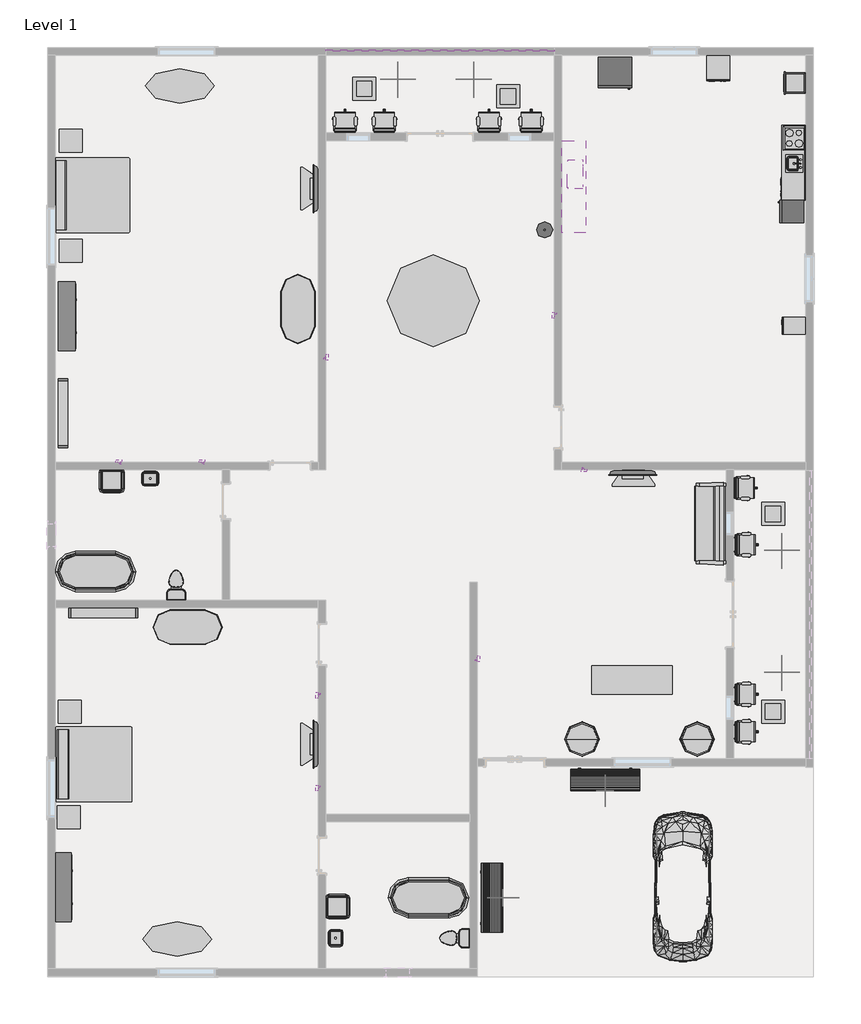
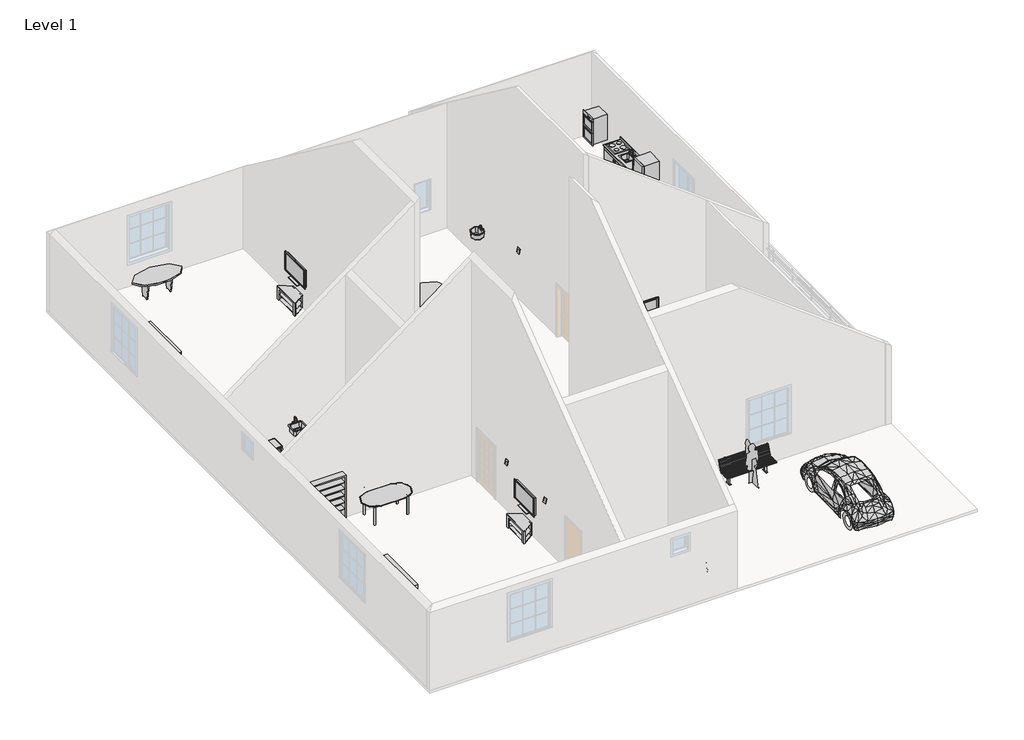
# One storey, part 2 of 2: 39 furniture elements, 20 proxies, 8 flow terminals, 8 geographic elements, 1 railing.
"""IFC4 building model written with IfcOpenShell, lengths in millimetres."""

from ifc_helpers import new_model, si_unit, point, frame, frame_2d, origin, place, context, project, spatial, circle_curve, trimmed, segment, composite_curve, outline, extrude, transform, mapped, element, save
from components import proxy_7e1014cc, proxy_a6faaae8, proxy_45b28599, proxy_19aded4c, kitchenette_medium_kitchenette_medium_844211aa, proxy_8a8d5ab2, proxy_8b8c2dc4, rpc_beetle_rpc_beetle_3ce7ba48, rpc_female_69e001fa, rpc_picture_frame_rpc_picture_frame_c25e3fe9, proxy_c523a7b7, proxy_9109806d, flow_terminal_871c2e40, flow_terminal_d49f872f, flow_terminal_62a433f7, toilet_domestic_3d_toilet_domestic_3d_f7549cf7, toilet_domestic_3d_toilet_domestic_3d_183bbd19, flow_terminal_b46ab875, furniture_1fc5af50, chair_task_arms_chair_task_arms_fa5a08ef, furniture_c6510c7c, counter_top_w_sink_hole_counter_top_w_sink_hole_22cae41e, furniture_7c473f12, furniture_c6fa4874, furniture_aff9b2fb, furniture_fdf74506, tv_stand_tv_stand_6ce107e5, furniture_b5c51a22, furniture_92191dda, furniture_2c34a4f9, furniture_5d3b8c6f, furniture_027a2ad9, furniture_5bc9ed15, furniture_c80d6d9c, geographic_element_235d1464, rpc_tree_conifer_chinese_juniper_7_1b9786cd, trash_can_trash_can_952d1acd

model = new_model("IFC4")

# Units and contexts
model_context = context("Model", 3, world=origin())
ifc_project = project(units=[si_unit("LENGTHUNIT", "METRE", prefix="MILLI")], contexts=[model_context])

# Site, building, storey
site = spatial("IfcSite", under=ifc_project)
building = spatial("IfcBuilding", under=site)
storey = spatial("IfcBuildingStorey", under=building, Name="Level 1", Elevation=0.0)

# Proxies
placement = place(None, origin())
proxy_shape = proxy_7e1014cc(model_context)
element("IfcBuildingElementProxy", 1, Name="18\" x 24\" x 34 1/2\"", ObjectType="18\" x 24\" x 34 1/2\"", at=placement, inside=storey, context=model_context, shape_type="MappedRepresentation", body=[
    mapped(proxy_shape, transform((4829.120864, 3840.6220575, 0.0), x_axis=(0.0, -1.0000000000000004, 0.0), y_axis=(1.0000000000000004, 0.0, 0.0), z_axis=(0.0, 0.0, 1.0))),
])
proxy_2_shape = proxy_a6faaae8(model_context)
element("IfcBuildingElementProxy", 2, Name="Cook Top-4 Unit2 : 22\" x 20\"", ObjectType="Cook Top-4 Unit2 : 22\" x 20\"", at=placement, inside=storey, context=model_context, shape_type="MappedRepresentation", body=[
    mapped(proxy_2_shape, transform((5095.5704288, 8500.2045891, 0.0), x_axis=(0.0, -1.0000000000000002, 0.0), y_axis=(1.0000000000000002, 0.0, 0.0), z_axis=(0.0, 0.0, 1.0))),
])
proxy_3_shape = proxy_45b28599(model_context)
element("IfcBuildingElementProxy", 3, Name="Dishwasher : 24\" x 24\" x 34\"", ObjectType="Dishwasher : 24\" x 24\" x 34\"", at=placement, inside=storey, context=model_context, shape_type="MappedRepresentation", body=[
    mapped(proxy_3_shape, transform((4803.720864, 7549.0220575, 0.0), x_axis=(0.0, -1.0000000000000002, 0.0), y_axis=(1.0000000000000002, 0.0, 0.0), z_axis=(0.0, 0.0, 1.0))),
])
proxy_4_shape = proxy_19aded4c(model_context)
element("IfcBuildingElementProxy", 4, Name="Dishwasher : 24\" x 26 1/4\" x 34 1/2\"", ObjectType="Dishwasher : 24\" x 26 1/4\" x 34 1/2\"", at=placement, inside=storey, context=model_context, shape_type="MappedRepresentation", body=[
    mapped(proxy_4_shape, transform((2706.6529603, 10068.9050243, 0.0), x_axis=(1.0, 0.0, 0.0), y_axis=(0.0, 1.0, 0.0), z_axis=(0.0, 0.0, 1.0))),
])
kitchenette_medium_kitchenette_medium_shape = kitchenette_medium_kitchenette_medium_844211aa(model_context)
element("IfcBuildingElementProxy", 5, Name="Kitchenette - Medium : Kitchenette - Medium", ObjectType="Kitchenette - Medium : Kitchenette - Medium", at=placement, inside=storey, context=model_context, shape_type="MappedRepresentation", body=[
    mapped(kitchenette_medium_kitchenette_medium_shape, transform((5400.3704288, 8176.042294, 0.0), x_axis=(0.0, -1.0000000000000002, 0.0), y_axis=(1.0000000000000002, 0.0, 0.0), z_axis=(0.0, 0.0, 1.0))),
])
proxy_5_shape = proxy_8a8d5ab2(model_context)
element("IfcBuildingElementProxy", 6, Name="Microwave : 30\" x 16\" x 18\"", ObjectType="Microwave : 30\" x 16\" x 18\"", at=placement, inside=storey, context=model_context, shape_type="MappedRepresentation", body=[
    mapped(proxy_5_shape, transform((-1061.410077, 7047.4117117, 914.4), x_axis=(0.0, 1.0000000000000004, 0.0), y_axis=(-1.0000000000000004, 0.0, 0.0), z_axis=(0.0, 0.0, 1.0))),
])
proxy_6_shape = proxy_8b8c2dc4(model_context)
element("IfcBuildingElementProxy", 7, Name="Oven Double-Built-in : 21 1/2\" x 39 1/4\" x 21\"", ObjectType="Oven Double-Built-in : 21 1/2\" x 39 1/4\" x 21\"", at=placement, inside=storey, context=model_context, shape_type="MappedRepresentation", body=[
    mapped(proxy_6_shape, transform((4979.9045698, 9925.5296617, 0.0), x_axis=(0.0, -1.0000000000000004, 0.0), y_axis=(1.0000000000000004, 0.0, 0.0), z_axis=(0.0, 0.0, 1.0))),
])
rpc_beetle_rpc_beetle_shape = rpc_beetle_rpc_beetle_3ce7ba48(model_context)
element("IfcBuildingElementProxy", 8, Name="RPC Beetle : RPC Beetle", ObjectType="RPC Beetle : RPC Beetle", at=placement, inside=storey, context=model_context, shape_type="MappedRepresentation", body=[
    mapped(rpc_beetle_rpc_beetle_shape, transform((2149.1704288, -12543.6954109, 0.0), x_axis=(1.0, 0.0, 0.0), y_axis=(0.0, 1.0, 0.0), z_axis=(0.0, 0.0, 1.0))),
])
rpc_female_shape = rpc_female_69e001fa(model_context)
element("IfcBuildingElementProxy", 9, Name="RPC Female", ObjectType="RPC Female", at=placement, inside=storey, context=model_context, shape_type="MappedRepresentation", body=[
    mapped(rpc_female_shape, transform((91.7704288, -8924.1954109, 0.0), x_axis=(1.0, 0.0, 0.0), y_axis=(0.0, 1.0, 0.0), z_axis=(0.0, 0.0, 1.0))),
])
element("IfcBuildingElementProxy", 10, Name="RPC Female", ObjectType="RPC Female", at=placement, inside=storey, context=model_context, shape_type="MappedRepresentation", body=[
    mapped(rpc_female_shape, transform((-2459.4958608, -11603.8954109, 0.0), x_axis=(0.0, 1.0, 0.0), y_axis=(-1.0, 0.0, 0.0), z_axis=(0.0, 0.0, 1.0))),
])
rpc_picture_frame_rpc_picture_frame_shape = rpc_picture_frame_rpc_picture_frame_c25e3fe9(model_context)
element("IfcBuildingElementProxy", 11, Name="RPC Picture Frame : RPC Picture Frame", ObjectType="RPC Picture Frame : RPC Picture Frame", at=placement, inside=storey, context=model_context, shape_type="MappedRepresentation", body=[
    mapped(rpc_picture_frame_rpc_picture_frame_shape, transform((-7502.8295712, -8696.2001393, 1828.8), x_axis=(0.0, -1.0000000000000002, 0.0), y_axis=(1.0000000000000002, 0.0, 0.0), z_axis=(0.0, 0.0, 1.0))),
])
element("IfcBuildingElementProxy", 12, Name="RPC Picture Frame : RPC Picture Frame", ObjectType="RPC Picture Frame : RPC Picture Frame", at=placement, inside=storey, context=model_context, shape_type="MappedRepresentation", body=[
    mapped(rpc_picture_frame_rpc_picture_frame_shape, transform((-12778.3105279, -72.2954109, 1828.8), x_axis=(-1.0000000000000004, 0.0, 0.0), y_axis=(0.0, -1.0000000000000004, 0.0), z_axis=(0.0, 0.0, 1.0))),
])
element("IfcBuildingElementProxy", 13, Name="RPC Picture Frame : RPC Picture Frame", ObjectType="RPC Picture Frame : RPC Picture Frame", at=placement, inside=storey, context=model_context, shape_type="MappedRepresentation", body=[
    mapped(rpc_picture_frame_rpc_picture_frame_shape, transform((-10576.3760013, -72.2954109, 1828.8), x_axis=(-1.0, 0.0, 0.0), y_axis=(0.0, -1.0, 0.0), z_axis=(0.0, 0.0, 1.0))),
])
element("IfcBuildingElementProxy", 14, Name="RPC Picture Frame : RPC Picture Frame", ObjectType="RPC Picture Frame : RPC Picture Frame", at=placement, inside=storey, context=model_context, shape_type="MappedRepresentation", body=[
    mapped(rpc_picture_frame_rpc_picture_frame_shape, transform((-7299.6295712, 2701.0709575, 1828.8), x_axis=(0.0, 1.0000000000000002, 0.0), y_axis=(-1.0000000000000002, 0.0, 0.0), z_axis=(0.0, 0.0, 1.0))),
])
element("IfcBuildingElementProxy", 15, Name="RPC Picture Frame : RPC Picture Frame", ObjectType="RPC Picture Frame : RPC Picture Frame", at=placement, inside=storey, context=model_context, shape_type="MappedRepresentation", body=[
    mapped(rpc_picture_frame_rpc_picture_frame_shape, transform((-1254.4295712, 3817.1261319, 1828.8), x_axis=(0.0, -1.0000000000000004, 0.0), y_axis=(1.0000000000000004, 0.0, 0.0), z_axis=(0.0, 0.0, 1.0))),
])
element("IfcBuildingElementProxy", 16, Name="RPC Picture Frame : RPC Picture Frame", ObjectType="RPC Picture Frame : RPC Picture Frame", at=placement, inside=storey, context=model_context, shape_type="MappedRepresentation", body=[
    mapped(rpc_picture_frame_rpc_picture_frame_shape, transform((-7502.8295712, -6241.8488853, 1828.8), x_axis=(0.0, -1.0000000000000004, 0.0), y_axis=(1.0000000000000004, 0.0, 0.0), z_axis=(0.0, 0.0, 1.0))),
])
element("IfcBuildingElementProxy", 17, Name="RPC Picture Frame : RPC Picture Frame", ObjectType="RPC Picture Frame : RPC Picture Frame", at=placement, inside=storey, context=model_context, shape_type="MappedRepresentation", body=[
    mapped(rpc_picture_frame_rpc_picture_frame_shape, transform((-468.7883262, -275.4954109, 1828.8), x_axis=(1.0, 0.0, 0.0), y_axis=(0.0, 1.0, 0.0), z_axis=(0.0, 0.0, 1.0))),
])
element("IfcBuildingElementProxy", 18, Name="RPC Picture Frame : RPC Picture Frame", ObjectType="RPC Picture Frame : RPC Picture Frame", at=placement, inside=storey, context=model_context, shape_type="MappedRepresentation", body=[
    mapped(rpc_picture_frame_rpc_picture_frame_shape, transform((-3286.4295712, -5279.3753115, 1828.8), x_axis=(0.0, 1.0000000000000002, 0.0), y_axis=(-1.0000000000000002, 0.0, 0.0), z_axis=(0.0, 0.0, 1.0))),
])
proxy_7_shape = proxy_c523a7b7(model_context)
element("IfcBuildingElementProxy", 19, Name="Refrigerator : 24\" x 25\" LH", ObjectType="Refrigerator : 24\" x 25\" LH", at=placement, inside=storey, context=model_context, shape_type="MappedRepresentation", body=[
    mapped(proxy_7_shape, transform((5049.9214573, 6563.4545891, 0.0), x_axis=(0.0, -1.0000000000000002, 0.0), y_axis=(1.0000000000000002, 0.0, 0.0), z_axis=(0.0, 0.0, 1.0))),
])
proxy_8_shape = proxy_9109806d(model_context)
element("IfcBuildingElementProxy", 20, Name="Refrigerator : 35\" x 32\" RH", ObjectType="Refrigerator : 35\" x 32\" RH", at=placement, inside=storey, context=model_context, shape_type="MappedRepresentation", body=[
    mapped(proxy_8_shape, transform((353.3194003, 10259.1545891, 0.0), x_axis=(1.0000000000000009, 0.0, 0.0), y_axis=(0.0, 1.0000000000000009, 0.0), z_axis=(0.0, 0.0, 1.0))),
])

# Flow terminals
flow_terminal_shape = flow_terminal_871c2e40(model_context)
element("IfcFlowTerminal", 21, ObjectType="Sink Kitchen-Island : 18\" x 18\"", at=placement, inside=storey, context=model_context, shape_type="MappedRepresentation", body=[
    mapped(flow_terminal_shape, transform((5093.2250277, 7842.7938296, -14.4), x_axis=(0.0, -1.0000000000000002, 0.0), y_axis=(1.0000000000000002, 0.0, 0.0), z_axis=(0.0, 0.0, 1.0))),
])
flow_terminal_2_shape = flow_terminal_d49f872f(model_context)
element("IfcFlowTerminal", 22, ObjectType="Sink Vanity-Round : 19\" x 19\"", at=placement, inside=storey, context=model_context, shape_type="MappedRepresentation", body=[
    mapped(flow_terminal_2_shape, transform((-1592.9717586, 6171.1563296, 609.6), x_axis=(0.0, -1.0000000000000004, 0.0), y_axis=(1.0000000000000004, 0.0, 0.0), z_axis=(0.0, 0.0, 1.0))),
])
flow_terminal_3_shape = flow_terminal_62a433f7(model_context)
element("IfcFlowTerminal", 23, ObjectType="Sink Vanity-Square : 20\" x 18\"", at=placement, inside=storey, context=model_context, shape_type="MappedRepresentation", body=[
    mapped(flow_terminal_3_shape, transform((-11963.5188118, -455.6408121, 609.6), x_axis=(1.0, 0.0, 0.0), y_axis=(0.0, 1.0, 0.0), z_axis=(0.0, 0.0, 1.0))),
])
element("IfcFlowTerminal", 24, ObjectType="Sink Vanity-Square : 20\" x 18\"", at=placement, inside=storey, context=model_context, shape_type="MappedRepresentation", body=[
    mapped(flow_terminal_3_shape, transform((-7094.0841701, -12686.3846515, 609.6), x_axis=(0.0, 1.0000000000000002, 0.0), y_axis=(-1.0000000000000002, 0.0, 0.0), z_axis=(0.0, 0.0, 1.0))),
])
toilet_domestic_3d_toilet_domestic_3d_shape = toilet_domestic_3d_toilet_domestic_3d_f7549cf7(model_context)
toilet_domestic_3d_toilet_domestic_3d_2_shape = toilet_domestic_3d_toilet_domestic_3d_183bbd19(model_context)
element("IfcFlowTerminal", 25, ObjectType="Toilet-Domestic-3D : Toilet-Domestic-3D", at=placement, inside=storey, context=model_context, shape_type="MappedRepresentation", body=[
    mapped(toilet_domestic_3d_toilet_domestic_3d_shape, transform((-11262.0295712, -3235.1993836, 0.0), x_axis=(-1.0000000000000004, 0.0, 0.0), y_axis=(0.0, -1.0000000000000004, 0.0), z_axis=(0.0, 0.0, 1.0))),
    mapped(toilet_domestic_3d_toilet_domestic_3d_2_shape, transform((-11262.0295712, -3235.1993836, 0.0), x_axis=(-1.0000000000000004, 0.0, 0.0), y_axis=(0.0, -1.0000000000000004, 0.0), z_axis=(0.0, 0.0, 1.0))),
])
element("IfcFlowTerminal", 26, ObjectType="Toilet-Domestic-3D : Toilet-Domestic-3D", at=placement, inside=storey, context=model_context, shape_type="MappedRepresentation", body=[
    mapped(toilet_domestic_3d_toilet_domestic_3d_shape, transform((-3984.3255986, -12670.6954109, 0.0), x_axis=(0.0, -1.0, 0.0), y_axis=(1.0, 0.0, 0.0), z_axis=(0.0, 0.0, 1.0))),
    mapped(toilet_domestic_3d_toilet_domestic_3d_2_shape, transform((-3984.3255986, -12670.6954109, 0.0), x_axis=(0.0, -1.0, 0.0), y_axis=(1.0, 0.0, 0.0), z_axis=(0.0, 0.0, 1.0))),
])
flow_terminal_4_shape = flow_terminal_b46ab875(model_context)
element("IfcFlowTerminal", 27, ObjectType="Tub-Free Standing-3D : 30\" x 60\"", at=placement, inside=storey, context=model_context, shape_type="MappedRepresentation", body=[
    mapped(flow_terminal_4_shape, transform((-13395.6295712, -2967.8954109, 0.0), x_axis=(0.0, 1.0000000000000002, 0.0), y_axis=(-1.0000000000000002, 0.0, 0.0), z_axis=(0.0, 0.0, 1.0))),
])
element("IfcFlowTerminal", 28, ObjectType="Tub-Free Standing-3D : 30\" x 60\"", at=placement, inside=storey, context=model_context, shape_type="MappedRepresentation", body=[
    mapped(flow_terminal_4_shape, transform((-4581.8295712, -11603.8954109, 0.0), x_axis=(0.0, -1.0, 0.0), y_axis=(1.0, 0.0, 0.0), z_axis=(0.0, 0.0, 1.0))),
])

# Furniture
furniture_shape = furniture_1fc5af50(model_context)
element("IfcFurniture", 29, ObjectType="Bed-Standard.0001 : King 78\" x 80\"", at=placement, inside=storey, context=model_context, shape_type="MappedRepresentation", body=[
    mapped(furniture_shape, transform((-13555.5246532, 6717.4160645, 0.0), x_axis=(0.0, 1.0, 0.0), y_axis=(-1.0, 0.0, 0.0), z_axis=(0.0, 0.0, 1.0))),
])
element("IfcFurniture", 30, ObjectType="Bed-Standard.0001 : King 78\" x 80\"", at=placement, inside=storey, context=model_context, shape_type="MappedRepresentation", body=[
    mapped(furniture_shape, transform((-13492.0246532, -8344.7839355, 0.0), x_axis=(0.0, 1.0000000000000002, 0.0), y_axis=(-1.0000000000000002, 0.0, 0.0), z_axis=(0.0, 0.0, 1.0))),
])
chair_task_arms_chair_task_arms_shape = chair_task_arms_chair_task_arms_fa5a08ef(model_context)
element("IfcFurniture", 31, ObjectType="Chair-Task Arms : Chair-Task Arms", at=placement, inside=storey, context=model_context, shape_type="MappedRepresentation", body=[
    mapped(chair_task_arms_chair_task_arms_shape, transform((3781.2245271, -2115.7045913, 0.0), x_axis=(0.0, -1.0000000000000004, 0.0), y_axis=(1.0000000000000004, 0.0, 0.0), z_axis=(0.0, 0.0, 1.0))),
])
element("IfcFurniture", 32, ObjectType="Chair-Task Arms : Chair-Task Arms", at=placement, inside=storey, context=model_context, shape_type="MappedRepresentation", body=[
    mapped(chair_task_arms_chair_task_arms_shape, transform((3755.8245271, -617.1045913, 0.0), x_axis=(0.0, -1.0000000000000016, 0.0), y_axis=(1.0000000000000016, 0.0, 0.0), z_axis=(0.0, 0.0, 1.0))),
])
element("IfcFurniture", 33, ObjectType="Chair-Task Arms : Chair-Task Arms", at=placement, inside=storey, context=model_context, shape_type="MappedRepresentation", body=[
    mapped(chair_task_arms_chair_task_arms_shape, transform((3781.2245271, -6078.1045913, 0.0), x_axis=(0.0, -1.0, 0.0), y_axis=(1.0, 0.0, 0.0), z_axis=(0.0, 0.0, 1.0))),
])
element("IfcFurniture", 34, ObjectType="Chair-Task Arms : Chair-Task Arms", at=placement, inside=storey, context=model_context, shape_type="MappedRepresentation", body=[
    mapped(chair_task_arms_chair_task_arms_shape, transform((3781.2245271, -7068.7045913, 0.0), x_axis=(0.0, -1.0000000000000007, 0.0), y_axis=(1.0000000000000007, 0.0, 0.0), z_axis=(0.0, 0.0, 1.0))),
])
element("IfcFurniture", 35, ObjectType="Chair-Task Arms : Chair-Task Arms", at=placement, inside=storey, context=model_context, shape_type="MappedRepresentation", body=[
    mapped(chair_task_arms_chair_task_arms_shape, transform((-6932.6203909, 8900.3586874, 0.0), x_axis=(1.0000000000000007, 0.0, 0.0), y_axis=(0.0, 1.0000000000000007, 0.0), z_axis=(0.0, 0.0, 1.0))),
])
element("IfcFurniture", 36, ObjectType="Chair-Task Arms : Chair-Task Arms", at=placement, inside=storey, context=model_context, shape_type="MappedRepresentation", body=[
    mapped(chair_task_arms_chair_task_arms_shape, transform((-5891.2203909, 8900.3586874, 0.0), x_axis=(1.0, 0.0, 0.0), y_axis=(0.0, 1.0, 0.0), z_axis=(0.0, 0.0, 1.0))),
])
element("IfcFurniture", 37, ObjectType="Chair-Task Arms : Chair-Task Arms", at=placement, inside=storey, context=model_context, shape_type="MappedRepresentation", body=[
    mapped(chair_task_arms_chair_task_arms_shape, transform((-3122.6203909, 8900.3586874, 0.0), x_axis=(1.0, 0.0, 0.0), y_axis=(0.0, 1.0, 0.0), z_axis=(0.0, 0.0, 1.0))),
])
element("IfcFurniture", 38, ObjectType="Chair-Task Arms : Chair-Task Arms", at=placement, inside=storey, context=model_context, shape_type="MappedRepresentation", body=[
    mapped(chair_task_arms_chair_task_arms_shape, transform((-2005.0203909, 8900.3586874, 0.0), x_axis=(1.0, 0.0, 0.0), y_axis=(0.0, 1.0, 0.0), z_axis=(0.0, 0.0, 1.0))),
])
furniture_2_shape = furniture_c6510c7c(model_context)
element("IfcFurniture", 39, ObjectType="Counter Top w Sink Hole : 24\" Depth", at=placement, inside=storey, context=model_context, shape_type="MappedRepresentation", body=[
    mapped(furniture_2_shape, transform((5400.3704288, 7642.642294, -14.4), x_axis=(0.0, -1.0000000000000002, 0.0), y_axis=(1.0000000000000002, 0.0, 0.0), z_axis=(0.0, 0.0, 1.0))),
])
counter_top_w_sink_hole_counter_top_w_sink_hole_shape = counter_top_w_sink_hole_counter_top_w_sink_hole_22cae41e(model_context)
element("IfcFurniture", 40, ObjectType="Counter Top w Sink Hole : Counter Top w Sink Hole", at=placement, inside=storey, context=model_context, shape_type="MappedRepresentation", body=[
    mapped(counter_top_w_sink_hole_counter_top_w_sink_hole_shape, transform((-1051.2295712, 7198.7668841, 914.4), x_axis=(0.0, 1.0000000000000002, 0.0), y_axis=(-1.0000000000000002, 0.0, 0.0), z_axis=(0.0, 0.0, 1.0))),
])
furniture_3_shape = furniture_7c473f12(model_context)
element("IfcFurniture", 41, ObjectType="Dresser : 72\" x 60\" x 18\"", at=placement, inside=storey, context=model_context, shape_type="MappedRepresentation", body=[
    mapped(furniture_3_shape, transform((-14520.7925253, 4057.6978489, 0.0), x_axis=(0.0, 1.0000000000000002, 0.0), y_axis=(-1.0000000000000002, 0.0, 0.0), z_axis=(0.0, 0.0, 1.0))),
])
element("IfcFurniture", 42, ObjectType="Dresser : 72\" x 60\" x 18\"", at=placement, inside=storey, context=model_context, shape_type="MappedRepresentation", body=[
    mapped(furniture_3_shape, transform((-14622.3925253, -11055.3021511, 0.0), x_axis=(0.0, 1.0000000000000002, 0.0), y_axis=(-1.0000000000000002, 0.0, 0.0), z_axis=(0.0, 0.0, 1.0))),
])
furniture_4_shape = furniture_c6fa4874(model_context)
element("IfcFurniture", 43, ObjectType="Shelving : 36\" x 10\" x 72\"", at=placement, inside=storey, context=model_context, shape_type="MappedRepresentation", body=[
    mapped(furniture_4_shape, transform((-14564.0295712, 1223.1045891, 0.0), x_axis=(0.0, 1.0000000000000002, 0.0), y_axis=(-1.0000000000000002, 0.0, 0.0), z_axis=(0.0, 0.0, 1.0))),
])
element("IfcFurniture", 44, ObjectType="Shelving : 36\" x 10\" x 72\"", at=placement, inside=storey, context=model_context, shape_type="MappedRepresentation", body=[
    mapped(furniture_4_shape, transform((-13192.4295712, -3755.2954109, 0.0), x_axis=(1.0, 0.0, 0.0), y_axis=(0.0, 1.0, 0.0), z_axis=(0.0, 0.0, 1.0))),
])
furniture_5_shape = furniture_aff9b2fb(model_context)
element("IfcFurniture", 45, ObjectType="Sofa-Pensi : 84\"", at=placement, inside=storey, context=model_context, shape_type="MappedRepresentation", body=[
    mapped(furniture_5_shape, transform((2608.6605927, -1419.2891609, 0.0), x_axis=(0.0, -1.0000000000000002, 0.0), y_axis=(1.0000000000000002, 0.0, 0.0), z_axis=(0.0, 0.0, 1.0))),
])
furniture_6_shape = furniture_fdf74506(model_context)
element("IfcFurniture", 46, ObjectType="TV - Flat Screen : 50\"", at=placement, inside=storey, context=model_context, shape_type="MappedRepresentation", body=[
    mapped(furniture_6_shape, transform((-7561.3681949, 7162.7600749, 914.4), x_axis=(0.0, -1.0000000000000002, 0.0), y_axis=(1.0000000000000002, 0.0, 0.0), z_axis=(0.0, 0.0, 1.0))),
])
element("IfcFurniture", 47, ObjectType="TV - Flat Screen : 50\"", at=placement, inside=storey, context=model_context, shape_type="MappedRepresentation", body=[
    mapped(furniture_6_shape, transform((-7561.3681949, -7543.8399251, 914.4), x_axis=(0.0, -1.0000000000000004, 0.0), y_axis=(1.0000000000000004, 0.0, 0.0), z_axis=(0.0, 0.0, 1.0))),
])
element("IfcFurniture", 48, ObjectType="TV - Flat Screen : 50\"", at=placement, inside=storey, context=model_context, shape_type="MappedRepresentation", body=[
    mapped(furniture_6_shape, transform((827.5517698, -356.5086217, 914.4), x_axis=(1.0000000000000007, 0.0, 0.0), y_axis=(0.0, 1.0000000000000007, 0.0), z_axis=(0.0, 0.0, 1.0))),
])
tv_stand_tv_stand_shape = tv_stand_tv_stand_6ce107e5(model_context)
element("IfcFurniture", 49, ObjectType="TV Stand : TV Stand", at=placement, inside=storey, context=model_context, shape_type="MappedRepresentation", body=[
    mapped(tv_stand_tv_stand_shape, transform((-7502.8295712, 7291.8925911, 0.0), x_axis=(0.0, -1.0, 0.0), y_axis=(1.0, 0.0, 0.0), z_axis=(0.0, 0.0, 1.0))),
])
element("IfcFurniture", 50, ObjectType="TV Stand : TV Stand", at=placement, inside=storey, context=model_context, shape_type="MappedRepresentation", body=[
    mapped(tv_stand_tv_stand_shape, transform((-7502.8295712, -7414.7074089, 0.0), x_axis=(0.0, -1.0000000000000004, 0.0), y_axis=(1.0000000000000004, 0.0, 0.0), z_axis=(0.0, 0.0, 1.0))),
])
element("IfcFurniture", 51, ObjectType="TV Stand : TV Stand", at=placement, inside=storey, context=model_context, shape_type="MappedRepresentation", body=[
    mapped(tv_stand_tv_stand_shape, transform((718.4347268, -256.9321966, 0.0), x_axis=(1.0000000000000007, 0.0, 0.0), y_axis=(0.0, 1.0000000000000007, 0.0), z_axis=(0.0, 0.0, 1.0))),
])
furniture_7_shape = furniture_b5c51a22(model_context)
element("IfcFurniture", 52, ObjectType="Table-Coffee : 24\" x 24\" x 24\"", at=placement, inside=storey, context=model_context, shape_type="MappedRepresentation", body=[
    mapped(furniture_7_shape, transform((-2491.8953379, 9509.8935112, 0.0), x_axis=(1.0, 0.0, 0.0), y_axis=(0.0, 1.0, 0.0), z_axis=(0.0, 0.0, 1.0))),
])
element("IfcFurniture", 53, ObjectType="Table-Coffee : 24\" x 24\" x 24\"", at=placement, inside=storey, context=model_context, shape_type="MappedRepresentation", body=[
    mapped(furniture_7_shape, transform((-6301.8953379, 9713.0935112, 0.0), x_axis=(1.0, 0.0, 0.0), y_axis=(0.0, 1.0, 0.0), z_axis=(0.0, 0.0, 1.0))),
])
element("IfcFurniture", 54, ObjectType="Table-Coffee : 24\" x 24\" x 24\"", at=placement, inside=storey, context=model_context, shape_type="MappedRepresentation", body=[
    mapped(furniture_7_shape, transform((4518.5046621, -1539.1064888, 0.0), x_axis=(1.0, 0.0, 0.0), y_axis=(0.0, 1.0, 0.0), z_axis=(0.0, 0.0, 1.0))),
])
element("IfcFurniture", 55, ObjectType="Table-Coffee : 24\" x 24\" x 24\"", at=placement, inside=storey, context=model_context, shape_type="MappedRepresentation", body=[
    mapped(furniture_7_shape, transform((4518.5046621, -6771.5064888, 0.0), x_axis=(1.0, 0.0, 0.0), y_axis=(0.0, 1.0, 0.0), z_axis=(0.0, 0.0, 1.0))),
])
furniture_8_shape = furniture_92191dda(model_context)
element("IfcFurniture", 56, ObjectType="Table-Dining : 30\" x 84\" x 22\"", at=placement, inside=storey, context=model_context, shape_type="MappedRepresentation", body=[
    mapped(furniture_8_shape, transform((821.2361955, -5742.8843331, 0.0), x_axis=(-1.0000000000000002, 0.0, 0.0), y_axis=(0.0, -1.0000000000000002, 0.0), z_axis=(0.0, 0.0, 1.0))),
])
furniture_9_shape = furniture_2c34a4f9(model_context)
element("IfcFurniture", 57, ObjectType="Table-Dining Oval : 36\" x 72\"", at=placement, inside=storey, context=model_context, shape_type="MappedRepresentation", body=[
    mapped(furniture_9_shape, transform((-10555.4098991, -4082.9970503, 0.0), x_axis=(1.0, 0.0, 0.0), y_axis=(0.0, 1.0, 0.0), z_axis=(0.0, 0.0, 1.0))),
])
element("IfcFurniture", 58, ObjectType="Table-Dining Oval : 36\" x 72\"", at=placement, inside=storey, context=model_context, shape_type="MappedRepresentation", body=[
    mapped(furniture_9_shape, transform((-8394.3279319, 4381.2832377, 0.0), x_axis=(0.0, 1.0000000000000002, 0.0), y_axis=(-1.0000000000000002, 0.0, 0.0), z_axis=(0.0, 0.0, 1.0))),
])
furniture_10_shape = furniture_5d3b8c6f(model_context)
element("IfcFurniture", 59, ObjectType="Table-Dining Round w Chairs : 84\" Diameter", at=placement, inside=storey, context=model_context, shape_type="MappedRepresentation", body=[
    mapped(furniture_10_shape, transform((-4558.5115384, 4379.7832776, 0.0), x_axis=(1.0, 0.0, 0.0), y_axis=(0.0, 1.0, 0.0), z_axis=(0.0, 0.0, 1.0))),
])
furniture_11_shape = furniture_027a2ad9(model_context)
element("IfcFurniture", 60, ObjectType="Table-Ellipse : 72\" x 36\"", at=placement, inside=storey, context=model_context, shape_type="MappedRepresentation", body=[
    mapped(furniture_11_shape, transform((-11160.4295712, 9884.5045891, 0.0), x_axis=(1.0, 0.0, 0.0), y_axis=(0.0, 1.0, 0.0), z_axis=(0.0, 0.0, 1.0))),
])
element("IfcFurniture", 61, ObjectType="Table-Ellipse : 72\" x 36\"", at=placement, inside=storey, context=model_context, shape_type="MappedRepresentation", body=[
    mapped(furniture_11_shape, transform((-11236.6295712, -12696.0954109, 0.0), x_axis=(1.0, 0.0, 0.0), y_axis=(0.0, 1.0, 0.0), z_axis=(0.0, 0.0, 1.0))),
])
furniture_12_shape = furniture_5bc9ed15(model_context)
element("IfcFurniture", 62, ObjectType="Table-Night Stand : 24\" x 24\" x 30\"", at=placement, inside=storey, context=model_context, shape_type="MappedRepresentation", body=[
    mapped(furniture_12_shape, transform((-14364.5632015, 8131.9045891, 0.0), x_axis=(1.0, 0.0, 0.0), y_axis=(0.0, 1.0, 0.0), z_axis=(0.0, 0.0, 1.0))),
])
element("IfcFurniture", 63, ObjectType="Table-Night Stand : 24\" x 24\" x 30\"", at=placement, inside=storey, context=model_context, shape_type="MappedRepresentation", body=[
    mapped(furniture_12_shape, transform((-14364.5632015, 5210.9045891, 0.0), x_axis=(1.0, 0.0, 0.0), y_axis=(0.0, 1.0, 0.0), z_axis=(0.0, 0.0, 1.0))),
])
element("IfcFurniture", 64, ObjectType="Table-Night Stand : 24\" x 24\" x 30\"", at=placement, inside=storey, context=model_context, shape_type="MappedRepresentation", body=[
    mapped(furniture_12_shape, transform((-14389.1605352, -6981.0954109, 0.0), x_axis=(1.0, 0.0, 0.0), y_axis=(0.0, 1.0, 0.0), z_axis=(0.0, 0.0, 1.0))),
])
element("IfcFurniture", 65, ObjectType="Table-Night Stand : 24\" x 24\" x 30\"", at=placement, inside=storey, context=model_context, shape_type="MappedRepresentation", body=[
    mapped(furniture_12_shape, transform((-14406.8887831, -9772.1398441, 0.0), x_axis=(1.0, 0.0, 0.0), y_axis=(0.0, 1.0, 0.0), z_axis=(0.0, 0.0, 1.0))),
])
furniture_13_shape = furniture_c80d6d9c(model_context)
element("IfcFurniture", 66, ObjectType="Table-Round : 36\" Diameter", at=placement, inside=storey, context=model_context, shape_type="MappedRepresentation", body=[
    mapped(furniture_13_shape, transform((2530.1704288, -7406.5454109, 0.0), x_axis=(1.0, 0.0, 0.0), y_axis=(0.0, 1.0, 0.0), z_axis=(0.0, 0.0, 1.0))),
])
element("IfcFurniture", 67, ObjectType="Table-Round : 36\" Diameter", at=placement, inside=storey, context=model_context, shape_type="MappedRepresentation", body=[
    mapped(furniture_13_shape, transform((-517.8295712, -7406.5454109, 0.0), x_axis=(1.0, 0.0, 0.0), y_axis=(0.0, 1.0, 0.0), z_axis=(0.0, 0.0, 1.0))),
])

# Geographic elements
geographic_element_shape = geographic_element_235d1464(model_context)
element("IfcGeographicElement", 68, ObjectType="Park Bench : 72\"", at=placement, inside=storey, context=model_context, shape_type="MappedRepresentation", body=[
    mapped(geographic_element_shape, transform((91.7704288, -8454.2954109, 0.0), x_axis=(1.0, 0.0, 0.0), y_axis=(0.0, 1.0, 0.0), z_axis=(0.0, 0.0, 1.0))),
])
element("IfcGeographicElement", 69, ObjectType="Park Bench : 72\"", at=placement, inside=storey, context=model_context, shape_type="MappedRepresentation", body=[
    mapped(geographic_element_shape, transform((-2930.8295712, -11603.8954109, 0.0), x_axis=(0.0, 1.0000000000000002, 0.0), y_axis=(-1.0000000000000002, 0.0, 0.0), z_axis=(0.0, 0.0, 1.0))),
])
rpc_tree_conifer_chinese_juniper_7_shape = rpc_tree_conifer_chinese_juniper_7_1b9786cd(model_context)
element("IfcGeographicElement", 70, ObjectType="RPC Tree - Conifer : Chinese Juniper - 7'", at=placement, inside=storey, context=model_context, shape_type="MappedRepresentation", body=[
    mapped(rpc_tree_conifer_chinese_juniper_7_shape, transform((4765.1737577, -5634.8954109, 0.0), x_axis=(1.0, 0.0, 0.0), y_axis=(0.0, 1.0, 0.0), z_axis=(0.0, 0.0, 1.0))),
])
element("IfcGeographicElement", 71, ObjectType="RPC Tree - Conifer : Chinese Juniper - 7'", at=placement, inside=storey, context=model_context, shape_type="MappedRepresentation", body=[
    mapped(rpc_tree_conifer_chinese_juniper_7_shape, transform((4765.1737577, -2409.0954109, 0.0), x_axis=(1.0, 0.0, 0.0), y_axis=(0.0, 1.0, 0.0), z_axis=(0.0, 0.0, 1.0))),
])
element("IfcGeographicElement", 72, ObjectType="RPC Tree - Conifer : Chinese Juniper - 7'", at=placement, inside=storey, context=model_context, shape_type="MappedRepresentation", body=[
    mapped(rpc_tree_conifer_chinese_juniper_7_shape, transform((-5394.8262423, 10062.3045891, 0.0), x_axis=(1.0, 0.0, 0.0), y_axis=(0.0, 1.0, 0.0), z_axis=(0.0, 0.0, 1.0))),
])
element("IfcGeographicElement", 73, ObjectType="RPC Tree - Conifer : Chinese Juniper - 7'", at=placement, inside=storey, context=model_context, shape_type="MappedRepresentation", body=[
    mapped(rpc_tree_conifer_chinese_juniper_7_shape, transform((-3388.2262423, 10062.3045891, 0.0), x_axis=(1.0, 0.0, 0.0), y_axis=(0.0, 1.0, 0.0), z_axis=(0.0, 0.0, 1.0))),
])
trash_can_trash_can_shape = trash_can_trash_can_952d1acd(model_context)
element("IfcGeographicElement", 74, ObjectType="Trash Can : Trash Can", at=placement, inside=storey, context=model_context, shape_type="MappedRepresentation", body=[
    mapped(trash_can_trash_can_shape, transform((-12963.8295712, -554.8954109, 0.0), x_axis=(1.0, 0.0, 0.0), y_axis=(0.0, 1.0, 0.0), z_axis=(0.0, 0.0, 1.0))),
])
element("IfcGeographicElement", 75, ObjectType="Trash Can : Trash Can", at=placement, inside=storey, context=model_context, shape_type="MappedRepresentation", body=[
    mapped(trash_can_trash_can_shape, transform((-6994.8295712, -11832.4954109, 0.0), x_axis=(1.0, 0.0, 0.0), y_axis=(0.0, 1.0, 0.0), z_axis=(0.0, 0.0, 1.0))),
])

# Railing
element("IfcRailing", 76, ObjectType="Guardrail - Pipe", at=placement, inside=storey, context=model_context, shape_type="SweptSolid", body=[
    extrude(outline(composite_curve([segment(trimmed(circle_curve(frame_2d((10824.3045891, 2114.55)), 19.05), [point((10843.3545891, 2114.55))], [point((10805.2545891, 2114.55))], False, "CARTESIAN"), True, "CONTINUOUS"), segment(trimmed(circle_curve(frame_2d((10824.3045891, 2114.55)), 19.05), [point((10805.2545891, 2114.55))], [point((10843.3545891, 2114.55))], False, "CARTESIAN"), True, "CONTINUOUS")], self_intersect=False)), frame((-7299.6295712, 0.0, 0.0), z_axis=(1.0, 0.0, 0.0), x_axis=(0.0, 1.0, 0.0)), (0.0, 0.0, 1.0), 6045.2),
    extrude(outline(composite_curve([segment(trimmed(circle_curve(frame_2d((10900.5045891, 2266.95)), 19.05), [point((10919.5545891, 2266.95))], [point((10881.4545891, 2266.95))], False, "CARTESIAN"), True, "CONTINUOUS"), segment(trimmed(circle_curve(frame_2d((10900.5045891, 2266.95)), 19.05), [point((10881.4545891, 2266.95))], [point((10919.5545891, 2266.95))], False, "CARTESIAN"), True, "CONTINUOUS")], self_intersect=False)), frame((-7299.6295712, 0.0, 0.0), z_axis=(1.0, 0.0, 0.0), x_axis=(0.0, 1.0, 0.0)), (0.0, 0.0, 1.0), 6045.2),
    extrude(outline(composite_curve([segment(trimmed(circle_curve(frame_2d((10900.5045891, 2120.9)), 12.7), [point((10887.8045891, 2120.9))], [point((10913.2045891, 2120.9))], False, "CARTESIAN"), True, "CONTINUOUS"), segment(trimmed(circle_curve(frame_2d((10900.5045891, 2120.9)), 12.7), [point((10913.2045891, 2120.9))], [point((10887.8045891, 2120.9))], False, "CARTESIAN"), True, "CONTINUOUS")], self_intersect=False)), frame((-7299.6295712, 0.0, 0.0), z_axis=(1.0, 0.0, 0.0), x_axis=(0.0, 1.0, 0.0)), (0.0, 0.0, 1.0), 6045.2),
    extrude(outline(composite_curve([segment(trimmed(circle_curve(frame_2d((10900.5045891, 1993.9)), 12.7), [point((10887.8045891, 1993.9))], [point((10913.2045891, 1993.9))], False, "CARTESIAN"), True, "CONTINUOUS"), segment(trimmed(circle_curve(frame_2d((10900.5045891, 1993.9)), 12.7), [point((10913.2045891, 1993.9))], [point((10887.8045891, 1993.9))], False, "CARTESIAN"), True, "CONTINUOUS")], self_intersect=False)), frame((-7299.6295712, 0.0, 0.0), z_axis=(1.0, 0.0, 0.0), x_axis=(0.0, 1.0, 0.0)), (0.0, 0.0, 1.0), 6045.2),
    extrude(outline(composite_curve([segment(trimmed(circle_curve(frame_2d((10900.5045891, 1866.9)), 12.7), [point((10887.8045891, 1866.9))], [point((10913.2045891, 1866.9))], False, "CARTESIAN"), True, "CONTINUOUS"), segment(trimmed(circle_curve(frame_2d((10900.5045891, 1866.9)), 12.7), [point((10913.2045891, 1866.9))], [point((10887.8045891, 1866.9))], False, "CARTESIAN"), True, "CONTINUOUS")], self_intersect=False)), frame((-7299.6295712, 0.0, 0.0), z_axis=(1.0, 0.0, 0.0), x_axis=(0.0, 1.0, 0.0)), (0.0, 0.0, 1.0), 6045.2),
    extrude(outline(composite_curve([segment(trimmed(circle_curve(frame_2d((10900.5045891, 1739.9)), 12.7), [point((10887.8045891, 1739.9))], [point((10913.2045891, 1739.9))], False, "CARTESIAN"), True, "CONTINUOUS"), segment(trimmed(circle_curve(frame_2d((10900.5045891, 1739.9)), 12.7), [point((10913.2045891, 1739.9))], [point((10887.8045891, 1739.9))], False, "CARTESIAN"), True, "CONTINUOUS")], self_intersect=False)), frame((-7299.6295712, 0.0, 0.0), z_axis=(1.0, 0.0, 0.0), x_axis=(0.0, 1.0, 0.0)), (0.0, 0.0, 1.0), 6045.2),
    extrude(outline(composite_curve([segment(trimmed(circle_curve(frame_2d((10900.5045891, 1612.9)), 12.7), [point((10887.8045891, 1612.9))], [point((10913.2045891, 1612.9))], False, "CARTESIAN"), True, "CONTINUOUS"), segment(trimmed(circle_curve(frame_2d((10900.5045891, 1612.9)), 12.7), [point((10913.2045891, 1612.9))], [point((10887.8045891, 1612.9))], False, "CARTESIAN"), True, "CONTINUOUS")], self_intersect=False)), frame((-7299.6295712, 0.0, 0.0), z_axis=(1.0, 0.0, 0.0), x_axis=(0.0, 1.0, 0.0)), (0.0, 0.0, 1.0), 6045.2),
    extrude(outline(composite_curve([segment(trimmed(circle_curve(frame_2d((10900.5045891, 1485.9)), 12.7), [point((10887.8045891, 1485.9))], [point((10913.2045891, 1485.9))], False, "CARTESIAN"), True, "CONTINUOUS"), segment(trimmed(circle_curve(frame_2d((10900.5045891, 1485.9)), 12.7), [point((10913.2045891, 1485.9))], [point((10887.8045891, 1485.9))], False, "CARTESIAN"), True, "CONTINUOUS")], self_intersect=False)), frame((-7299.6295712, 0.0, 0.0), z_axis=(1.0, 0.0, 0.0), x_axis=(0.0, 1.0, 0.0)), (0.0, 0.0, 1.0), 6045.2),
    extrude(outline(composite_curve([segment(trimmed(circle_curve(frame_2d((10900.5045891, 1358.9)), 12.7), [point((10887.8045891, 1358.9))], [point((10913.2045891, 1358.9))], False, "CARTESIAN"), True, "CONTINUOUS"), segment(trimmed(circle_curve(frame_2d((10900.5045891, 1358.9)), 12.7), [point((10913.2045891, 1358.9))], [point((10887.8045891, 1358.9))], False, "CARTESIAN"), True, "CONTINUOUS")], self_intersect=False)), frame((-7299.6295712, 0.0, 0.0), z_axis=(1.0, 0.0, 0.0), x_axis=(0.0, 1.0, 0.0)), (0.0, 0.0, 1.0), 6045.2),
    extrude(outline(composite_curve([segment(trimmed(circle_curve(frame_2d((-6131.2295712, 10900.5045891)), 12.7), [point((-6131.2295712, 10887.8045891))], [point((-6131.2295712, 10913.2045891))], False, "CARTESIAN"), True, "CONTINUOUS"), segment(trimmed(circle_curve(frame_2d((-6131.2295712, 10900.5045891)), 12.7), [point((-6131.2295712, 10913.2045891))], [point((-6131.2295712, 10887.8045891))], False, "CARTESIAN"), True, "CONTINUOUS")], self_intersect=False)), frame((0.0, 0.0, 1219.2), z_axis=(0.0, 0.0, 1.0), x_axis=(1.0, 0.0, 0.0)), (0.0, 0.0, 1.0), 1028.7),
    extrude(outline(composite_curve([segment(trimmed(circle_curve(frame_2d((-4912.0295712, 10900.5045891)), 12.7), [point((-4912.0295712, 10887.8045891))], [point((-4912.0295712, 10913.2045891))], False, "CARTESIAN"), True, "CONTINUOUS"), segment(trimmed(circle_curve(frame_2d((-4912.0295712, 10900.5045891)), 12.7), [point((-4912.0295712, 10913.2045891))], [point((-4912.0295712, 10887.8045891))], False, "CARTESIAN"), True, "CONTINUOUS")], self_intersect=False)), frame((0.0, 0.0, 1219.2), z_axis=(0.0, 0.0, 1.0), x_axis=(1.0, 0.0, 0.0)), (0.0, 0.0, 1.0), 1028.7),
    extrude(outline(composite_curve([segment(trimmed(circle_curve(frame_2d((-3692.8295712, 10900.5045891)), 12.7), [point((-3692.8295712, 10887.8045891))], [point((-3692.8295712, 10913.2045891))], False, "CARTESIAN"), True, "CONTINUOUS"), segment(trimmed(circle_curve(frame_2d((-3692.8295712, 10900.5045891)), 12.7), [point((-3692.8295712, 10913.2045891))], [point((-3692.8295712, 10887.8045891))], False, "CARTESIAN"), True, "CONTINUOUS")], self_intersect=False)), frame((0.0, 0.0, 1219.2), z_axis=(0.0, 0.0, 1.0), x_axis=(1.0, 0.0, 0.0)), (0.0, 0.0, 1.0), 1028.7),
    extrude(outline(composite_curve([segment(trimmed(circle_curve(frame_2d((-2473.6295712, 10900.5045891)), 12.7), [point((-2473.6295712, 10887.8045891))], [point((-2473.6295712, 10913.2045891))], False, "CARTESIAN"), True, "CONTINUOUS"), segment(trimmed(circle_curve(frame_2d((-2473.6295712, 10900.5045891)), 12.7), [point((-2473.6295712, 10913.2045891))], [point((-2473.6295712, 10887.8045891))], False, "CARTESIAN"), True, "CONTINUOUS")], self_intersect=False)), frame((0.0, 0.0, 1219.2), z_axis=(0.0, 0.0, 1.0), x_axis=(1.0, 0.0, 0.0)), (0.0, 0.0, 1.0), 1028.7),
    extrude(outline(composite_curve([segment(trimmed(circle_curve(frame_2d((-7286.9295712, 10900.5045891)), 12.7), [point((-7286.9295712, 10887.8045891))], [point((-7286.9295712, 10913.2045891))], False, "CARTESIAN"), True, "CONTINUOUS"), segment(trimmed(circle_curve(frame_2d((-7286.9295712, 10900.5045891)), 12.7), [point((-7286.9295712, 10913.2045891))], [point((-7286.9295712, 10887.8045891))], False, "CARTESIAN"), True, "CONTINUOUS")], self_intersect=False)), frame((0.0, 0.0, 1219.2), z_axis=(0.0, 0.0, 1.0), x_axis=(1.0, 0.0, 0.0)), (0.0, 0.0, 1.0), 1028.7),
    extrude(outline(composite_curve([segment(trimmed(circle_curve(frame_2d((-1267.1295712, 10900.5045891)), 12.7), [point((-1267.1295712, 10887.8045891))], [point((-1267.1295712, 10913.2045891))], False, "CARTESIAN"), True, "CONTINUOUS"), segment(trimmed(circle_curve(frame_2d((-1267.1295712, 10900.5045891)), 12.7), [point((-1267.1295712, 10913.2045891))], [point((-1267.1295712, 10887.8045891))], False, "CARTESIAN"), True, "CONTINUOUS")], self_intersect=False)), frame((0.0, 0.0, 1219.2), z_axis=(0.0, 0.0, 1.0), x_axis=(1.0, 0.0, 0.0)), (0.0, 0.0, 1.0), 1028.7),
])

save(model, "model.ifc")

# Revit data of these elements
# Type "18\" x 24\" x 34 1/2\""
#   Label = "T"
#   Assembly Code = "E1090400"
#   Depth = 2' - 0"
#   Height = 2' - 10 1/2"
#   Width = 1' - 6"
#   Panel Face Material = Plastic, Opaque Black
#   Trach Compact. Material = Steel, Paint Finish, Ivory, Matte
#   Default Elevation = 0
# Type "Cook Top-4 Unit2 : 22\" x 20\""
#   Depth = 1' - 8"
#   Width = 1' - 10"
#   Burner Material = Steel, Chrome Plated
#   Cooktop Material = Steel, Polished
#   Default Elevation = 0
#   Assembly Code = ""
# Type "Dishwasher : 24\" x 24\" x 34\""
#   Label = "DW"
#   Assembly Code = "E1090400"
#   Depth = 2' - 0"
#   Height = 2' - 10"
#   Width = 2' - 0"
#   Dishwasher Material = Steel, Paint Finish, Ivory, Glossy
#   Panel Face Material = Plastic, Opaque Black
#   Default Elevation = 0
# Type "Dishwasher : 24\" x 26 1/4\" x 34 1/2\""
#   Label = "DW"
#   Assembly Code = "E1090400"
#   Depth = 2' - 2 1/4"
#   Height = 2' - 10 1/2"
#   Width = 2' - 0"
#   Dishwasher Material = Steel, Paint Finish, Ivory, Glossy
#   Panel Face Material = Plastic, Opaque Black
#   Default Elevation = 0
# Type "Kitchenette - Medium : Kitchenette - Medium"
#   Assembly Code = "E1090400"
#   Counter Length = 6' - 6"
#   Cabinet Width = 4' - 6"
#   Cabinet Height = 2' - 10 1/2"
#   Cabinet Depth = 2' - 0"
#   Toe Depth = 0' - 3"
#   Toe Height = 0' - 3 1/2"
#   Cabinet Material = Cabinets
#   Door/Drawer Material = Cabinets
#   Handle Material = Cabinets - Handles
#   Default Elevation = 0
# Type "Microwave : 30\" x 16\" x 18\""
#   Assembly Code = "E1090400"
#   Depth = 1' - 4"
#   Height = 1' - 6"
#   Width = 2' - 6"
#   Microwave Material = Laminate, Ivory, Matte
#   Default Elevation = 0
# Type "Oven Double-Built-in : 21 1/2\" x 39 1/4\" x 21\""
#   Label = "OVEN"
#   Assembly Code = "E1090400"
#   Depth = 1' - 9"
#   Height = 3' - 3 1/4"
#   Width = 1' - 9 1/2"
#   Oven Material = Metal - Stainless Steel, Polished
#   Default Elevation = 0
# Type "RPC Beetle : RPC Beetle"
#   built-in parameter 1005195 = "RPC-16-0U6E-L4EG-ENH1-J3KF-SVEL-0TX4-C0"
#   Height = 0
# Type "RPC Female"
#   built-in parameter 1005195 = "RPC-8-FXA2-QQQ0-UGV2-6"
#   Height = 0
# Type "RPC Picture Frame : RPC Picture Frame"
#   built-in parameter 1005198 = "{2, 15},{39, RPC-16-8M5E-0H3T-F0AH-3U0K-JLQ7-G28B-AU},{1, 0},{1, 0},{2, 19},{1, 8},{5, Color},{1, 0},{1, 0},{3, 0.8},{3, 0.8},{3, 0.8},{1, 8},{7, BBoxMin},{1, 0},{1, 0},{1, 0},{1, 0},{1, 0},{1, 8},{7, BBoxMax},{1, 0},{1, 0},{1, 0},{1, 0},{1, 0},{2, 11},{9, RPCTypeId},{1, 0},{1, 0},{39, RPC-16-8M5E-0H3T-F0AH-3U0K-JLQ7-G28B-AU},{1, 6},{14, RPCPlantHeight},{1, 0},{1, 0},{5, 0.625},{2, 11},{7, keyword},{1, 0},{1, 0},{33, :RPCs:Office Clutter:Geometry:RPC},{2, 11},{8, category},{1, 0},{1, 0},{14, Office Clutter},{2, 11},{12, LocalizedUID},{1, 0},{1, 0},{13, Picture Frame},{2, 14},{6, Height},{1, 0},{1, 0},{5, 0.625},{1, 2},{16, Cast Reflections},{1, 0},{1, 0},{1, 0},{1, 2},{8, Portrait},{1, 0},{1, 0},{1, 1},{1, 2},{5, Stand},{1, 0},{1, 0},{1, 1},{2, 11},{10, RPCL_Frame},{1, 0},{1, 0},{5, Frame},{1, 4},{14, Frame Material},{1, 0},{1, 0},{1, 0},{2, 11},{12, RPCL_Picture},{1, 0},{1, 0},{7, Picture},{2, 11},{15, Picture Preview},{1, 0},{1, 0},{65, __RPC:/object data/textures/object/Photo/Photo0/textures/Portrait},{2, 11},{17, i_Picture Preview},{1, 0},{1, 0},{0, },{1, 2},{18, Use Custom Picture},{1, 0},{1, 0},{1, 0},{2, 11},{17, Picture File Name},{1, 0},{1, 0},{0, },{21, assetlibrary_base.fbx},{1, 5},"
#   built-in parameter 1005195 = "RPC-16-8M5E-0H3T-F0AH-3U0K-JLQ7-G28B-AU"
#   Height = 0
# Type "Refrigerator : 24\" x 25\" LH"
#   Label = "REF."
#   Assembly Code = "E1090400"
#   Depth = 2' - 0 3/4"
#   Handle = 0' - 1 1/2"
#   Height = 5' - 3 1/2"
#   Rear Clearance = 0' - 2"
#   Top Door Height = 1' - 8"
#   Width = 1' - 11 1/2"
#   Material = Steel, Paint Finish, Ivory, Glossy
#   Default Elevation = 0
# Type "Refrigerator : 35\" x 32\" RH"
#   Label = "REF."
#   Assembly Code = "E1090400"
#   Depth = 2' - 7 3/4"
#   Handle = 2' - 7"
#   Height = 5' - 10"
#   Rear Clearance = 0' - 2"
#   Top Door Height = 1' - 8"
#   Width = 2' - 10 1/2"
#   Material = Steel, Paint Finish, Ivory, Glossy
#   Default Elevation = 0
# Type "Sink Kitchen-Island : 18\" x 18\""
#   Assembly Code = "D2010410"
#   Counter Height = 3' - 0"
#   Depth = 1' - 6"
#   Width = 1' - 6"
#   Faucet Material = Steel, Polished
#   Sink Material = Steel, Polished
#   Default Elevation = 0
# Type "Sink Vanity-Round : 19\" x 19\""
#   Assembly Code = "D2010400"
#   Top Of Counter = 2' - 7"
#   Basin Material = Porcelain, Linen
#   Faucet Material = Steel, Polished
#   Default Elevation = 0
# Type "Sink Vanity-Square : 20\" x 18\""
#   Assembly Code = "D2010400"
#   Counter Height = 2' - 7"
#   Depth = 1' - 6"
#   Width = 1' - 8"
#   Basin Material = Porcelain, Linen
#   Faucet Material = Steel, Polished
#   Default Elevation = 0
# Type "Toilet-Domestic-3D : Toilet-Domestic-3D"
#   Assembly Code = "D2010110"
#   Toilet - Bowl/Basin Material = Porcelain, Linen
#   Toilet - Seat Material = Laminate, Linen, Matte
#   Default Elevation = 0
# Type "Tub-Free Standing-3D : 30\" x 60\""
#   Assembly Code = "D2010110"
#   Height = 2' - 6"
#   Length = 7' - 0"
#   Width = 3' - 6"
#   Tub Material = Porcelain, Ivory
#   Default Elevation = 0
# Type "Bed-Standard.0001 : King 78\" x 80\""
#   Assembly Code = "E2020200"
#   Length = 6' - 8"
#   Width = 6' - 6"
#   Leg Material = Steel, Chrome Plated
#   Mattress Material = Linen, White
#   Default Elevation = 0
# Type "Chair-Task Arms : Chair-Task Arms"
#   Assembly Code = "E2020200"
#   Base Material = Plastic, Opaque Black
#   Caster Material = Plastic, Opaque Black
#   Seat/Back Material = Textile - Slate Blue
#   Default Elevation = 0
# Type "Counter Top w Sink Hole : 24\" Depth"
#   Assembly Code = "C1030400"
#   Counter Thickness = 0' - 1 1/2"
#   Depth = 2' - 1"
#   Height = 3' - 0"
#   Length [instance default] = 8' - 0"
#   Sink Location [instance default] = 2' - 0"
#   Sink Location To Wall [instance default] = 0' - 6"
#   Sink Opening Depth [instance default] = 1' - 3"
#   Sink Opening Width [instance default] = 2' - 3"
#   Counter Top Material = none
#   Default Elevation = 0
# Type "Counter Top w Sink Hole : Counter Top w Sink Hole"
#   Assembly Code = "C1030400"
#   Counter Thickness = 0' - 1 1/2"
#   Depth = 2' - 1"
#   Height = 3' - 0"
#   Length [instance default] = 8' - 0"
#   Sink Location [instance default] = 2' - 0"
#   Sink Location To Wall [instance default] = 0' - 6"
#   Sink Opening Depth [instance default] = 1' - 3"
#   Sink Opening Width [instance default] = 2' - 3"
#   Counter Top Material = none
#   Default Elevation = 0
# Type "Dresser : 72\" x 60\" x 18\""
#   Assembly Code = "E2020200"
#   Depth = 1' - 6"
#   Height = 5' - 0"
#   Width = 6' - 0"
#   Dresser Material = Laminate - Ivory, Glossy
#   Drawer Material = Laminate, Ivory, Matte
#   Knob Material = Cherry
#   Default Elevation = 0
# Type "Shelving : 36\" x 10\" x 72\""
#   Assembly Code = "E2020200"
#   Depth = 0' - 10"
#   Height = 6' - 0"
#   Width = 6' - 0"
#   Shelving Unit Material = Birch
#   Default Elevation = 0
# Type "Sofa-Pensi : 84\""
#   Assembly Code = "E2020200"
#   Length = 7' - 0"
#   Frame Material = Cherry
#   Seat Material = Linen, Beige
#   Feet Material = Steel, Chrome Plated
#   Default Elevation = 0
# Type "TV - Flat Screen : 50\""
#   SinAng = 0' - 0.0193"
#   L = 3' - 7.57782"
#   H = 2' - 0.51477"
#   Thickness = 0' - 4.33071"
#   Diagonal = 4' - 2"
#   CosAng = 0' - 0.03431"
#   Stand [instance default] = yes
#   Default Elevation = 0
# Type "TV Stand : TV Stand"
#   Depth = 1' - 6"
#   Width = 3' - 8"
#   Height = 1' - 7 1/2"
#   Finish = Melamine - Gray
#   Default Elevation = 0
# Type "Table-Coffee : 24\" x 24\" x 24\""
#   Assembly Code = "E2020200"
#   Height = 2' - 0"
#   Length = 2' - 0"
#   Width = 2' - 0"
#   Top Material = none
#   Frame Material = none
#   Default Elevation = 0
# Type "Table-Dining : 30\" x 84\" x 22\""
#   Assembly Code = "E2020200"
#   Height = 1' - 10"
#   Length = 7' - 0"
#   Width = 2' - 6"
#   Base Material = Steel, Chrome Plated
#   Top Material = Glass - Clear, Grey
#   Default Elevation = 0
# Type "Table-Dining Oval : 36\" x 72\""
#   Assembly Code = "E2020200"
#   Length = 6' - 0"
#   Width = 3' - 0"
#   Base Material = Steel, Chrome Plated
#   Top Material = Glass - Clear, Grey
#   Default Elevation = 0
#   Description = (empty or 0)
# Type "Table-Dining Round w Chairs : 84\" Diameter"
#   Assembly Code = "E2020200"
#   Radius = 4' - 0"
#   Diameter = 8' - 0"
#   Height = 2' - 6"
#   Chairs = 10
#   Base Material = Pine
#   Top Material = Laminate, Linen, Matte
#   Default Elevation = 0
# Type "Table-Ellipse : 72\" x 36\""
#   Assembly Code = "E2020200"
#   Half Width = 1' - 6"
#   Half Length = 3' - 0"
#   Height = 2' - 6"
#   Length = 6' - 0"
#   Width = 3' - 0"
#   Base Material = Birch
#   Top Material = Laminate - Black
#   Default Elevation = 0
# Type "Table-Night Stand : 24\" x 24\" x 30\""
#   Assembly Code = "E2020200"
#   Depth = 2' - 0"
#   Height = 2' - 6"
#   Width = 2' - 0"
#   Base Material = Birch
#   Top Material = Laminate, Ivory, Matte
#   Default Elevation = 0
# Type "Table-Round : 36\" Diameter"
#   Assembly Code = "E2020200"
#   Base Radius = 0' - 10"
#   Height = 2' - 6"
#   Radius = 1' - 6"
#   Base Material = Steel, Chrome Plated
#   Top Material = Birch
#   Default Elevation = 0
# Type "Park Bench : 72\""
#   Length = 6' - 0"
#   Seat Material = Wood - Teak
#   Frame Material = Steel, Paint Finish, Dark Gray, Matte
# Type "RPC Tree - Conifer : Chinese Juniper - 7'"
#   built-in parameter 1005198 = "{2, 15},{39, RPC-16-FUM3-UUQ0-UBF0-N000-ST1L-LVER-AU},{1, 0},{1, 0},{2, 13},{1, 8},{5, Color},{1, 0},{1, 0},{3, 0.8},{3, 0.8},{3, 0.8},{1, 8},{7, BBoxMin},{1, 0},{1, 0},{1, 0},{1, 0},{1, 0},{1, 8},{7, BBoxMax},{1, 0},{1, 0},{1, 0},{1, 0},{1, 0},{2, 11},{9, RPCTypeId},{1, 0},{1, 0},{39, RPC-16-FUM3-UUQ0-UBF0-N000-ST1L-LVER-AU},{1, 6},{14, RPCPlantHeight},{1, 0},{1, 0},{1, 7},{2, 11},{7, keyword},{1, 0},{1, 0},{34, :RPCs:Trees [General]:Geometry:RPC},{2, 11},{8, category},{1, 0},{1, 0},{15, Trees [General]},{2, 11},{12, LocalizedUID},{1, 0},{1, 0},{15, Chinese Juniper},{2, 14},{6, Height},{1, 0},{1, 0},{1, 7},{1, 2},{16, Cast Reflections},{1, 0},{1, 0},{1, 0},{1, 2},{12, Cast Shadows},{1, 0},{1, 0},{1, 1},{1, 2},{9, Lock View},{1, 0},{1, 0},{1, 0},{1, 4},{5, ViewC},{1, 0},{1, 0},{1, 0},{21, assetlibrary_base.fbx},{1, 5},"
#   built-in parameter 1005195 = "RPC-16-FUM3-UUQ0-UBF0-N000-ST1L-LVER-AU"
#   Type Comments = "Chinese Juniper"
#   Assembly Code = "G2050500"
#   Height = 7' - 0"
#   Description = (empty or 0)
#   Default Elevation = 0
# Type "Trash Can : Trash Can"
#   Assembly Code = "G2040900"
# Type "Guardrail - Pipe"
#   Assembly Code = "C2010400"
#   built-in parameter 1008612 = 0.0416667 (stored number, unit not read)
#   built-in parameter 1008611 = 0.0833333 (stored number, unit not read)
#   built-in parameter 1008609 = 4 (stored number, unit not read)
#   built-in parameter 1008604 = 0.166667 (stored number, unit not read)
#   built-in parameter 1008603 = 0.166667 (stored number, unit not read)
#   Railing Height = 3' - 6"
#   built-in parameter 1008630 = 2
#   built-in parameter 1008610 = 1
#   built-in parameter 1008605 = 1
#   built-in parameter 1008618 = Baluster - Round : 1"
# Element 1 (IfcBuildingElementProxy, "18\" x 24\" x 34 1/2\"")
#   Phase Created = New Construction
#   Materials on its faces: "Steel, Paint Finish, Ivory, Matte", "Plastic, Opaque Black"
# Element 2 (IfcBuildingElementProxy, "Cook Top-4 Unit2 : 22\" x 20\"")
#   Phase Created = New Construction
#   Materials on its faces: "Steel, Chrome Plated", "Steel, Polished"
# Element 3 (IfcBuildingElementProxy, "Dishwasher : 24\" x 24\" x 34\"")
#   Phase Created = New Construction
#   Materials on its faces: "Steel, Paint Finish, Ivory, Glossy", "Plastic, Opaque Black"
# Element 4 (IfcBuildingElementProxy, "Dishwasher : 24\" x 26 1/4\" x 34 1/2\"")
#   Phase Created = New Construction
#   Materials on its faces: "Steel, Paint Finish, Ivory, Glossy", "Plastic, Opaque Black"
# Element 5 (IfcBuildingElementProxy, "Kitchenette - Medium : Kitchenette - Medium")
#   Phase Created = New Construction
#   Materials on its faces: "Cabinets", "Cabinets - Handles"
# Element 6 (IfcBuildingElementProxy, "Microwave : 30\" x 16\" x 18\"")
#   Phase Created = New Construction
#   Materials on its faces: "Laminate, Ivory, Matte", "Glass"
# Element 7 (IfcBuildingElementProxy, "Oven Double-Built-in : 21 1/2\" x 39 1/4\" x 21\"")
#   Phase Created = New Construction
#   Materials on its faces: "Steel", "Metal - Stainless Steel, Polished", "Glass"
# Element 8 (IfcBuildingElementProxy, "RPC Beetle : RPC Beetle")
#   Phase Created = New Construction
# Elements 9, 10 (IfcBuildingElementProxy, "RPC Female")
#   Phase Created = New Construction
# Elements 11, 12, 13, 14, 15, 16, 17, 18 (IfcBuildingElementProxy, "RPC Picture Frame : RPC Picture Frame")
#   Phase Created = New Construction
# Element 19 (IfcBuildingElementProxy, "Refrigerator : 24\" x 25\" LH")
#   Phase Created = New Construction
#   Materials on its faces: "Steel, Paint Finish, Ivory, Glossy", "Steel, Chrome Plated"
# Element 20 (IfcBuildingElementProxy, "Refrigerator : 35\" x 32\" RH")
#   Phase Created = New Construction
#   Materials on its faces: "Steel, Paint Finish, Ivory, Glossy", "Steel, Chrome Plated"
# Element 21 (IfcFlowTerminal, "Sink Kitchen-Island : 18\" x 18\"")
#   Mark = "8"
#   Phase Created = New Construction
#   Materials on its faces: "Steel, Polished"
# Element 22 (IfcFlowTerminal, "Sink Vanity-Round : 19\" x 19\"")
#   Mark = "9"
#   Phase Created = New Construction
#   Materials on its faces: "Porcelain, Linen", "Steel, Polished"
# Element 23 (IfcFlowTerminal, "Sink Vanity-Square : 20\" x 18\"")
#   Mark = "3"
#   Phase Created = New Construction
